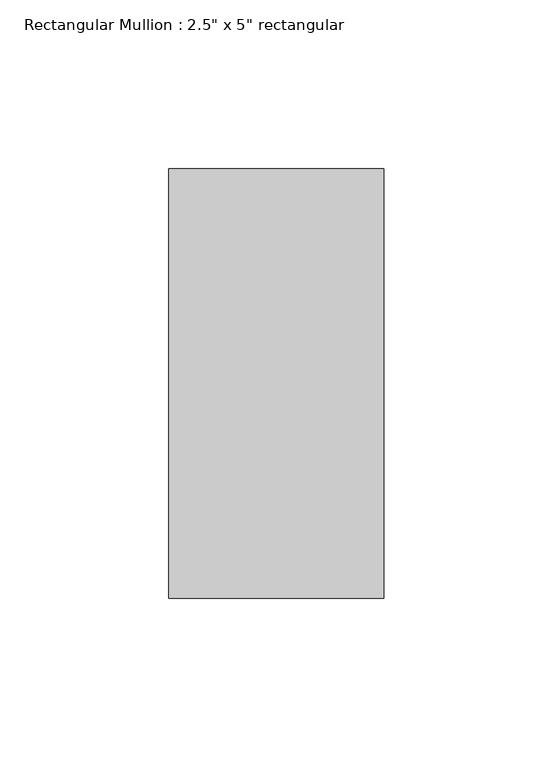
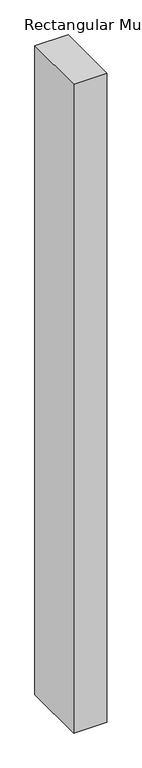
"""IFC4 building model written with IfcOpenShell, lengths in millimetres: member geometry."""

from ifc_helpers import new_model, si_unit, frame, origin, place, context, project, spatial, polyline, outline, extrude, source, transform, mapped, element, save


def member_65750824(model_context):
    return source(origin(), model_context, "Body", "SweptSolid", [
        extrude(outline(polyline([(0.0, 63.5), (0.0, -63.5), (-63.5, -63.5), (-63.5, 63.5), (0.0, 63.5)])), frame((0.0, 0.0, -1301.75), z_axis=(0.0, 0.0, 1.0), x_axis=(1.0, 0.0, 0.0)), (0.0, 0.0, 1.0), 1301.75),
    ])


if __name__ == "__main__":
    model = new_model("IFC4")
    model_context = context("Model", 3, world=origin())
    ifc_project = project(units=[si_unit("LENGTHUNIT", "METRE", prefix="MILLI")], contexts=[model_context])
    site = spatial("IfcSite", under=ifc_project)
    building = spatial("IfcBuilding", under=site)
    placement = place(None, origin())
    member_shape = member_65750824(model_context)
    element("IfcMember", 1, ObjectType="Rectangular Mullion : 2.5\" x 5\" rectangular", at=placement, inside=building, context=model_context, shape_type="MappedRepresentation", body=[
        mapped(member_shape, transform((0.0, 0.0, 0.0), x_axis=(1.0, 0.0, 0.0), y_axis=(0.0, 1.0, 0.0), z_axis=(0.0, 0.0, 1.0))),
    ])
    save(model, "model.ifc")

# Revit data of these elements
# Type "Rectangular Mullion : 2.5\" x 5\" rectangular"
#   built-in parameter 1007304 = 0.416667 (stored number, unit not read)
#   built-in parameter 1007301 = 0.104167 (stored number, unit not read)
#   built-in parameter 1007300 = 0.104167 (stored number, unit not read)
# Element 1 (IfcMember, "Rectangular Mullion : 2.5\" x 5\" rectangular")
#   Materials on its faces: "Aluminum"
# Materials
#   "Aluminum": class "Metal", colour RGB 247 247 247, transparency 0, Description = "Aluminum 6061", Cost = 0
